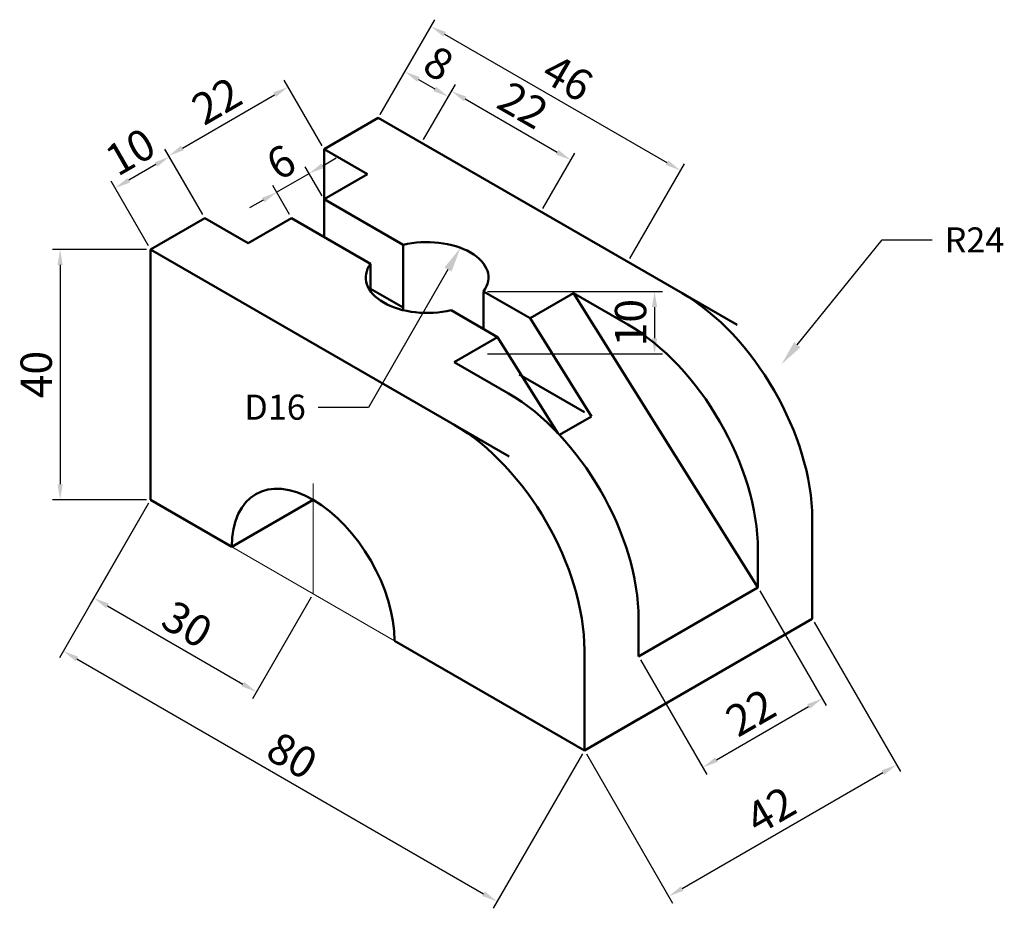
# Model space of a CAD drawing. Units: millimetres. Extents: x 2885 to 3042, y 1127 to 1268.
import ezdxf
from ezdxf import colors
from ezdxf.entities.mleader import LeaderData, LeaderLine
from ezdxf.math import Vec2, Vec3

# ---------------------------------------------------------------- set-up
doc = ezdxf.new("R2010")
doc.units = ezdxf.units.MM
doc.linetypes.add('CENTER', pattern=[50.8, 31.75, -6.35, 6.35, -6.35])
for name, color, linetype, lineweight in [('M-CNTR', 1, 'CENTER', 18), ('M-DIMS', 2, 'Continuous', 25), ('M-OUTL', 7, 'Continuous', 50), ('M-TEXT', 3, 'Continuous', 25)]:
    doc.layers.add(name, color=color, linetype=linetype, lineweight=lineweight)
doc.styles.get("Standard").update_dxf_attribs({"font": 'arial.ttf'})
doc.dimstyles.new('ISO-25', dxfattribs={"dimtxt": 5, "dimasz": 2.5, "dimexe": 1.25, "dimexo": 0.625, "dimtad": 1, "dimtxsty": 'Standard', "dimcen": 2.5, "dimadec": 0, "dimazin": 0, "dimtfac": 1, "dimtmove": 0, "dimatfit": 3, "dimfxl": 1, "dimarcsym": 0})

# ---------------------------------------------------------------- blocks, each defined once
blk = doc.blocks.new('*D1')
at = {"layer": 'Defpoints', "color": 0, "transparency": 16777216}
for p in [(2905.82, 1231.8), (2891.39, 1191.8), (2905.82, 1191.8)]:
    blk.add_point(p, dxfattribs=at)
at = {"layer": 'M-DIMS', "color": 0, "lineweight": -2, "transparency": 16777216}
for p, q in [((2905.19, 1231.8), (2890.14, 1231.8)), ((2891.39, 1229.3), (2891.39, 1194.3)), ((2905.19, 1191.8), (2890.14, 1191.8))]:
    blk.add_line(p, q, dxfattribs=at)
at = {"layer": 'M-DIMS', "color": 0, "transparency": 16777216}
for points in [[(2890.97, 1229.3), (2891.8, 1229.3), (2891.39, 1231.8)], [(2890.97, 1194.3), (2891.8, 1194.3), (2891.39, 1191.8)]]:
    blk.add_solid(points, dxfattribs=at)
at = {"layer": 'M-DIMS', "color": 0, "transparency": 16777216, "insert": (2888.21, 1211.8), "char_height": 5, "attachment_point": 5, "rotation": 90}
blk.add_mtext('40', dxfattribs=at)
blk = doc.blocks.new('*D2')
at = {"layer": 'Defpoints', "color": 0, "transparency": 16777216}
for p in [(2905.82, 1191.8), (2931.8, 1176.8), (2922.75, 1161.12)]:
    blk.add_point(p, dxfattribs=at)
at = {"layer": 'M-DIMS', "color": 0, "lineweight": -2, "transparency": 16777216}
for p, q in [((2905.5, 1191.26), (2896.14, 1175.04)), ((2931.48, 1176.26), (2922.12, 1160.04)), ((2898.93, 1174.87), (2920.58, 1162.37))]:
    blk.add_line(p, q, dxfattribs=at)
at = {"layer": 'M-DIMS', "color": 0, "transparency": 16777216}
for points in [[(2899.14, 1175.23), (2898.72, 1174.51), (2896.77, 1176.12)], [(2920.79, 1162.73), (2920.37, 1162.01), (2922.75, 1161.12)]]:
    blk.add_solid(points, dxfattribs=at)
at = {"layer": 'M-DIMS', "color": 0, "transparency": 16777216, "insert": (2911.35, 1171.38), "char_height": 5, "attachment_point": 5, "rotation": 330}
blk.add_mtext('30', dxfattribs=at)
blk = doc.blocks.new('*D3')
at = {"layer": 'Defpoints', "color": 0, "transparency": 16777216}
for p in [(2905.82, 1191.8), (2975.1, 1151.8), (2961.16, 1127.66)]:
    blk.add_point(p, dxfattribs=at)
at = {"layer": 'M-DIMS', "color": 0, "lineweight": -2, "transparency": 16777216}
for p, q in [((2905.5, 1191.26), (2891.26, 1166.58)), ((2894.05, 1166.41), (2959, 1128.91)), ((2974.79, 1151.26), (2960.54, 1126.58))]:
    blk.add_line(p, q, dxfattribs=at)
at = {"layer": 'M-DIMS', "color": 0, "transparency": 16777216}
for points in [[(2894.25, 1166.77), (2893.84, 1166.05), (2891.88, 1167.66)], [(2959.21, 1129.27), (2958.79, 1128.55), (2961.16, 1127.66)]]:
    blk.add_solid(points, dxfattribs=at)
at = {"layer": 'M-DIMS', "color": 0, "transparency": 16777216, "insert": (2928.11, 1150.41), "char_height": 5, "attachment_point": 5, "rotation": 330}
blk.add_mtext('80', dxfattribs=at)
blk = doc.blocks.new('*D4')
at = {"layer": 'Defpoints', "color": 0, "transparency": 16777216}
for p in [(3002.81, 1177.8), (2983.76, 1166.8), (3013.05, 1160.06)]:
    blk.add_point(p, dxfattribs=at)
at = {"layer": 'M-DIMS', "color": 0, "lineweight": -2, "transparency": 16777216}
for p, q in [((3003.12, 1177.26), (3013.68, 1158.97)), ((2984.07, 1166.26), (2994.63, 1147.97)), ((2996.17, 1150.31), (3010.89, 1158.81))]:
    blk.add_line(p, q, dxfattribs=at)
at = {"layer": 'M-DIMS', "color": 0, "transparency": 16777216}
for points in [[(3010.68, 1159.17), (3011.1, 1158.44), (3013.05, 1160.06)], [(2995.96, 1150.67), (2996.37, 1149.94), (2994, 1149.06)]]:
    blk.add_solid(points, dxfattribs=at)
at = {"layer": 'M-DIMS', "color": 0, "transparency": 16777216, "insert": (3001.96, 1157.27), "char_height": 5, "attachment_point": 5, "rotation": 30}
blk.add_mtext('22', dxfattribs=at)
blk = doc.blocks.new('*D5')
at = {"layer": 'Defpoints', "color": 0, "transparency": 16777216}
for p in [(3011.47, 1172.8), (2975.1, 1151.8), (3024.93, 1149.49)]:
    blk.add_point(p, dxfattribs=at)
at = {"layer": 'M-DIMS', "color": 0, "lineweight": -2, "transparency": 16777216}
for p, q in [((3011.78, 1172.26), (3025.55, 1148.4)), ((2975.41, 1151.26), (2989.18, 1127.4)), ((2990.72, 1129.74), (3022.76, 1148.24))]:
    blk.add_line(p, q, dxfattribs=at)
at = {"layer": 'M-DIMS', "color": 0, "transparency": 16777216}
for points in [[(3022.56, 1148.6), (3022.97, 1147.88), (3024.93, 1149.49)], [(2990.51, 1130.1), (2990.93, 1129.38), (2988.56, 1128.49)]]:
    blk.add_solid(points, dxfattribs=at)
at = {"layer": 'M-DIMS', "color": 0, "transparency": 16777216, "insert": (3005.17, 1141.7), "char_height": 5, "attachment_point": 5, "rotation": 30}
blk.add_mtext('42', dxfattribs=at)
blk = doc.blocks.new('*D6')
at = {"layer": 'Defpoints', "color": 0, "transparency": 16777216}
for p in [(2900.17, 1241.58), (2914.48, 1236.8), (2905.82, 1231.8)]:
    blk.add_point(p, dxfattribs=at)
at = {"layer": 'M-DIMS', "color": 0, "lineweight": -2, "transparency": 16777216}
for p, q in [((2914.16, 1237.34), (2908.2, 1247.66)), ((2906.66, 1245.33), (2902.33, 1242.83)), ((2905.5, 1232.34), (2899.54, 1242.66))]:
    blk.add_line(p, q, dxfattribs=at)
at = {"layer": 'M-DIMS', "color": 0, "transparency": 16777216}
for points in [[(2906.45, 1245.69), (2906.87, 1244.97), (2908.83, 1246.58)], [(2902.12, 1243.19), (2902.54, 1242.47), (2900.17, 1241.58)]]:
    blk.add_solid(points, dxfattribs=at)
at = {"layer": 'M-DIMS', "color": 0, "transparency": 16777216, "insert": (2902.91, 1246.83), "char_height": 5, "attachment_point": 5, "rotation": 30}
blk.add_mtext('10', dxfattribs=at)
blk = doc.blocks.new('*D7')
at = {"layer": 'Defpoints', "color": 0, "transparency": 16777216}
for p in [(2927.79, 1257.73), (2933.53, 1247.8), (2914.48, 1236.8)]:
    blk.add_point(p, dxfattribs=at)
at = {"layer": 'M-DIMS', "color": 0, "lineweight": -2, "transparency": 16777216}
for p, q in [((2933.22, 1248.34), (2927.17, 1258.82)), ((2910.9, 1247.98), (2925.63, 1256.48)), ((2914.16, 1237.34), (2908.11, 1247.82))]:
    blk.add_line(p, q, dxfattribs=at)
at = {"layer": 'M-DIMS', "color": 0, "transparency": 16777216}
for points in [[(2925.42, 1256.85), (2925.83, 1256.12), (2927.79, 1257.73)], [(2910.69, 1248.35), (2911.11, 1247.62), (2908.74, 1246.73)]]:
    blk.add_solid(points, dxfattribs=at)
at = {"layer": 'M-DIMS', "color": 0, "transparency": 16777216, "insert": (2916.7, 1254.95), "char_height": 5, "attachment_point": 5, "rotation": 30}
blk.add_mtext('22', dxfattribs=at)
blk = doc.blocks.new('*D8')
at = {"layer": 'Defpoints', "color": 0, "transparency": 16777216}
for p in [(2931.15, 1243.91), (2933.53, 1239.8), (2928.33, 1236.8)]:
    blk.add_point(p, dxfattribs=at)
at = {"layer": 'M-DIMS', "color": 0, "lineweight": -2, "transparency": 16777216}
for p, q in [((2933.32, 1245.16), (2935.48, 1246.41)), ((2925.96, 1240.91), (2931.15, 1243.91)), ((2933.22, 1240.34), (2930.53, 1244.99)), ((2928.02, 1237.34), (2925.33, 1241.99)), ((2923.79, 1239.66), (2921.63, 1238.41))]:
    blk.add_line(p, q, dxfattribs=at)
at = {"layer": 'M-DIMS', "color": 0, "transparency": 16777216}
for points in [[(2933.11, 1245.52), (2933.53, 1244.8), (2931.15, 1243.91)], [(2923.58, 1240.02), (2924, 1239.3), (2925.96, 1240.91)]]:
    blk.add_solid(points, dxfattribs=at)
at = {"layer": 'M-DIMS', "color": 0, "transparency": 16777216, "insert": (2926.97, 1245.16), "char_height": 5, "attachment_point": 5, "rotation": 30}
blk.add_mtext('6', dxfattribs=at)
blk = doc.blocks.new('*D9')
at = {"layer": 'Defpoints', "color": 0, "transparency": 16777216}
for p in [(2942.19, 1252.8), (2990.45, 1244.39), (2982.03, 1229.8)]:
    blk.add_point(p, dxfattribs=at)
at = {"layer": 'M-DIMS', "color": 0, "lineweight": -2, "transparency": 16777216}
for p, q in [((2942.5, 1253.34), (2951.24, 1268.47)), ((2952.78, 1266.14), (2988.28, 1245.64)), ((2982.34, 1230.34), (2991.07, 1245.47))]:
    blk.add_line(p, q, dxfattribs=at)
at = {"layer": 'M-DIMS', "color": 0, "transparency": 16777216}
for points in [[(2952.99, 1266.5), (2952.57, 1265.78), (2950.61, 1267.39)], [(2988.49, 1246), (2988.08, 1245.28), (2990.45, 1244.39)]]:
    blk.add_solid(points, dxfattribs=at)
at = {"layer": 'M-DIMS', "color": 0, "transparency": 16777216, "insert": (2972.12, 1258.64), "char_height": 5, "attachment_point": 5, "rotation": 330}
blk.add_mtext('46', dxfattribs=at)
blk = doc.blocks.new('*D10')
at = {"layer": 'Defpoints', "color": 0, "transparency": 16777216}
for p in [(2953.37, 1256.17), (2942.19, 1252.8), (2949.12, 1248.8)]:
    blk.add_point(p, dxfattribs=at)
at = {"layer": 'M-DIMS', "color": 0, "lineweight": -2, "transparency": 16777216}
for p, q in [((2942.5, 1253.34), (2947.07, 1261.25)), ((2948.61, 1258.92), (2951.21, 1257.42)), ((2949.43, 1249.34), (2954, 1257.25))]:
    blk.add_line(p, q, dxfattribs=at)
at = {"layer": 'M-DIMS', "color": 0, "transparency": 16777216}
for points in [[(2948.82, 1259.28), (2948.4, 1258.56), (2946.45, 1260.17)], [(2951.42, 1257.78), (2951, 1257.06), (2953.37, 1256.17)]]:
    blk.add_solid(points, dxfattribs=at)
at = {"layer": 'M-DIMS', "color": 0, "transparency": 16777216, "insert": (2951.5, 1260.92), "char_height": 5, "attachment_point": 5, "rotation": 330}
blk.add_mtext('8', dxfattribs=at)
blk = doc.blocks.new('*D11')
at = {"layer": 'Defpoints', "color": 0, "transparency": 16777216}
for p in [(2949.12, 1248.8), (2972.94, 1246.06), (2968.17, 1237.8)]:
    blk.add_point(p, dxfattribs=at)
at = {"layer": 'M-DIMS', "color": 0, "lineweight": -2, "transparency": 16777216}
for p, q in [((2949.43, 1249.34), (2954.51, 1258.14)), ((2956.05, 1255.81), (2970.77, 1247.31)), ((2968.48, 1238.34), (2973.56, 1247.14))]:
    blk.add_line(p, q, dxfattribs=at)
at = {"layer": 'M-DIMS', "color": 0, "transparency": 16777216}
for points in [[(2956.26, 1256.17), (2955.84, 1255.44), (2953.88, 1257.06)], [(2970.98, 1247.67), (2970.56, 1246.94), (2972.94, 1246.06)]]:
    blk.add_solid(points, dxfattribs=at)
at = {"layer": 'M-DIMS', "color": 0, "transparency": 16777216, "insert": (2964.98, 1254.27), "char_height": 5, "attachment_point": 5, "rotation": 330}
blk.add_mtext('22', dxfattribs=at)
blk = doc.blocks.new('*D12')
at = {"layer": 'Defpoints', "color": 0, "transparency": 16777216}
for p in [(2959, 1225.09), (2959, 1215.09), (2986.3, 1215.09)]:
    blk.add_point(p, dxfattribs=at)
at = {"layer": 'M-DIMS', "color": 0, "lineweight": -2, "transparency": 16777216}
for p, q in [((2959.63, 1225.09), (2987.55, 1225.09)), ((2986.3, 1222.59), (2986.3, 1217.59)), ((2959.63, 1215.09), (2987.55, 1215.09))]:
    blk.add_line(p, q, dxfattribs=at)
at = {"layer": 'M-DIMS', "color": 0, "transparency": 16777216}
for points in [[(2985.88, 1222.59), (2986.72, 1222.59), (2986.3, 1225.09)], [(2985.88, 1217.59), (2986.72, 1217.59), (2986.3, 1215.09)]]:
    blk.add_solid(points, dxfattribs=at)
at = {"layer": 'M-DIMS', "color": 0, "transparency": 16777216, "insert": (2983.12, 1220.09), "char_height": 5, "attachment_point": 5, "rotation": 90}
blk.add_mtext('10', dxfattribs=at)

msp = doc.modelspace()

# ---------------------------------------------------------------- linework, layer by layer
at = {"layer": 'M-CNTR'}
for p, q in [((2931.796, 1176.797), (2931.796, 1194.398)), ((2918.806, 1184.297), (2944.787, 1169.297))]:
    msp.add_line(p, q, dxfattribs=at)
at = {"layer": 'M-OUTL'}
for p, q in [((2942.189, 1252.797), (2933.528, 1247.797)), ((2999.471, 1219.725), (2942.189, 1252.797)), ((2933.528, 1247.797), (2940.457, 1243.797)), ((2933.528, 1239.797), (2933.528, 1247.797)), ((2940.457, 1243.797), (2933.528, 1239.797)), ((2933.528, 1239.797), (2946.158, 1232.505)), ((2933.528, 1233.797), (2933.528, 1239.797)), ((2905.816, 1231.797), (2914.476, 1236.797)), ((2914.476, 1236.797), (2921.404, 1232.797)), ((2921.404, 1232.797), (2928.332, 1236.797)), ((2928.332, 1236.797), (2940.962, 1229.505)), ((2928.332, 1236.797), (2940.962, 1229.505)), ((2905.816, 1191.797), (2905.816, 1231.797)), ((2905.816, 1231.797), (2963.098, 1198.725)), ((2946.158, 1232.505), (2946.158, 1222.089)), ((2940.962, 1225.089), (2940.962, 1229.505)), ((2946.158, 1222.505), (2940.962, 1225.505)), ((2959.004, 1225.089), (2966.437, 1220.797)), ((2959.004, 1225.089), (2959.004, 1219.089)), ((2966.437, 1220.797), (2973.366, 1224.797)), ((2973.366, 1224.797), (3002.81, 1177.797)), ((2982.026, 1219.797), (2973.366, 1224.797)), ((2953.807, 1222.089), (2961.241, 1217.797)), ((2976.252, 1205.13), (2966.437, 1220.797)), ((2954.313, 1213.797), (2961.241, 1217.797)), ((2970.85, 1202.459), (2961.241, 1217.797)), ((2962.973, 1208.797), (2954.313, 1213.797)), ((2964.705, 1211.797), (2975.098, 1205.797)), ((2976.252, 1205.13), (2971.124, 1202.169)), ((2905.816, 1191.797), (2918.806, 1184.297)), ((2918.806, 1184.297), (2905.816, 1191.797)), ((2918.806, 1184.297), (2931.796, 1191.797)), ((3011.471, 1172.797), (3011.471, 1188.797)), ((3002.81, 1183.797), (3002.81, 1177.797)), ((2983.758, 1166.797), (3002.81, 1177.797)), ((3002.81, 1177.797), (2995.882, 1173.797)), ((2975.098, 1151.797), (3011.471, 1172.797)), ((2983.758, 1172.797), (2983.758, 1166.797)), ((2975.098, 1151.797), (2944.787, 1169.297)), ((2975.098, 1151.797), (2975.098, 1167.797)), ((2975.098, 1151.797), (2975.098, 1161.797)), ((2975.098, 1151.797), (2983.758, 1156.797))]:
    msp.add_line(p, q, dxfattribs=at)
for centre, major_axis, start_param, end_param in [((2949.983, 1227.297), (-9.798, 0), 9.0237766, 11.3965757), ((2949.983, 1227.297), (-9.798, 0), 5.8821839, 8.254983), ((2990.686, 1200.797), (-14.697, 25.456), 3.9269908, 5.4977871), ((2982.026, 1195.797), (14.697, -25.456), 0.7853982, 2.3561945), ((2962.973, 1184.797), (14.697, -25.456), 0.7853982, 2.3561945), ((2954.313, 1179.797), (-14.697, 25.456), 3.9269908, 5.4977871), ((2931.796, 1176.797), (9.186, -15.91), 0.7853982, 3.9269908)]:
    msp.add_ellipse(centre, major_axis=major_axis, ratio=0.5773503, start_param=start_param, end_param=end_param, dxfattribs=at)

# ---------------------------------------------------------------- dimensions: what is measured, and where the dimension line sits
at = {"layer": 'M-DIMS'}
for p1, p2, distance, picture, middle in [((2942.189, 1252.797), (2982.026, 1229.797), 16.846, '*D9', (2972.119, 1258.638)), ((2942.189, 1252.797), (2949.117, 1248.797), 8.513, '*D10', (2951.498, 1260.922)), ((2914.476, 1236.797), (2933.528, 1247.797), 11.475, '*D7', (2916.697, 1254.95)), ((2949.117, 1248.797), (2968.169, 1237.797), 9.536, '*D11', (2964.979, 1254.27)), ((2914.476, 1236.797), (2905.816, 1231.797), -11.298, '*D6', (2902.908, 1246.833)), ((2928.332, 1236.797), (2933.528, 1239.797), 4.75, '*D8', (2926.966, 1245.163)), ((2905.816, 1231.797), (2905.816, 1191.797), -14.429, '*D1', (2888.209, 1211.797)), ((2959.004, 1225.089), (2959.004, 1215.089), 27.296, '*D12', (2983.122, 1220.089)), ((2905.816, 1191.797), (2975.098, 1151.797), -27.87, '*D3', (2928.111, 1150.413)), ((2905.816, 1191.797), (2931.796, 1176.797), -18.1, '*D2', (2911.346, 1171.376)), ((2983.758, 1166.797), (3002.81, 1177.797), -20.486, '*D4', (3001.96, 1157.271)), ((2975.098, 1151.797), (3011.471, 1172.797), -26.916, '*D5', (3005.175, 1141.702))]:
    dim = msp.add_aligned_dim(p1=p1, p2=p2, distance=distance, dimstyle='ISO-25', override={"dimclrd": 0, "dimclre": 0, "dimclrt": 0}, dxfattribs=at)
    dim.commit()
    dim.dimension.update_dxf_attribs({"geometry": picture, "text_midpoint": middle})

# ---------------------------------------------------------------- leaders
at = {"layer": 'M-TEXT'}
ml = msp.add_multileader_mtext('Standard', dxfattribs=at)
ml.set_content('R24', color=256)
ml.set_leader_properties()
ml.build(insert=Vec2(0, 0))
ctx = ml.context
ctx.base_point, ctx.plane_origin = Vec3(3030.625, 1233.303), Vec3(3006.582, 1213.458)
notes = []
notes.append((ctx, [(0, (1, 1, 0), (3022.625, 1233.303), (1, 0), 8, [(0, [(3006.582, 1213.458)], 0, [])])]))
ctx.mtext.insert, ctx.mtext.flow_direction = Vec3(3032.625, 1235.303), 5
ml = msp.add_multileader_mtext('Standard', dxfattribs=at)
ml.set_content('D16', color=256)
ml.set_leader_properties()
ml.build(insert=Vec2(0, 0))
ctx = ml.context
ctx.base_point, ctx.plane_origin = Vec3(2919.043, 1206.564), Vec3(2955.316, 1232.042)
ctx.text_align_type = 2
notes.append((ctx, [(0, (1, 1, 0), (2940.606, 1206.564), (-1, 0), 8, [(0, [(2955.316, 1232.042)], 0, [])])]))
ctx.mtext.insert, ctx.mtext.alignment, ctx.mtext.flow_direction = Vec3(2930.606, 1208.598), 3, 5
for ctx, leaders in notes:
    for number, flags, end, landing, length, lines in leaders:
        leader = LeaderData()
        leader.index, (leader.has_last_leader_line, leader.has_dogleg_vector, leader.attachment_direction) = number, flags
        leader.last_leader_point, leader.dogleg_vector, leader.dogleg_length = Vec3(end), Vec3(landing), length
        for number, points, colour, breaks in lines:
            line = LeaderLine()
            line.index, line.vertices, line.color, line.breaks = number, Vec3.list(points), colors.encode_raw_color(colour), breaks
            leader.lines.append(line)
        ctx.leaders.append(leader)

doc.saveas('drawing.dxf')
